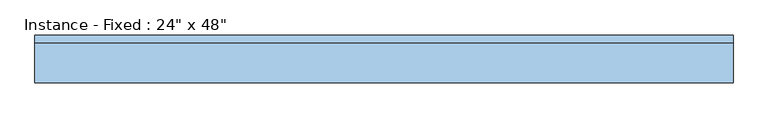
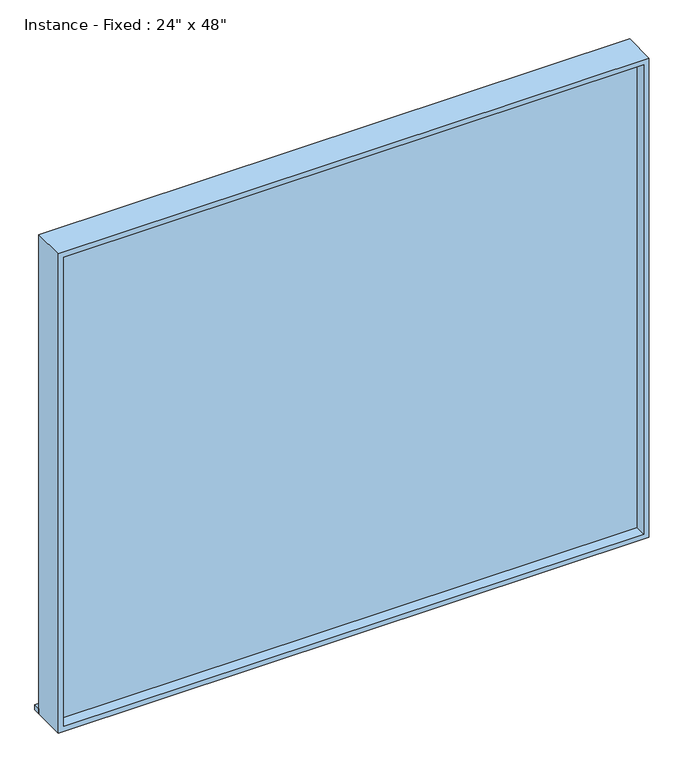
"""IFC4 building model written with IfcOpenShell, lengths in millimetres: window geometry."""

from ifc_helpers import new_model, si_unit, frame, origin, place, context, project, spatial, polyline, outline, extrude, source, transform, mapped, element, save


def window_88b07bfa(model_context):
    return source(origin(), model_context, "Body", "SweptSolid", [
        extrude(outline(polyline([(-1104.9, 127.0), (1028.7, 127.0), (1028.7, 101.6), (-1104.9, 101.6), (-1104.9, 127.0)])), frame((0.0, 0.0, 914.4), z_axis=(0.0, 0.0, 1.0), x_axis=(1.0, 0.0, 0.0)), (0.0, 0.0, 1.0), 19.05),
        extrude(outline(polyline([(1009.65, 22.225), (-1085.85, 22.225), (-1085.85, 34.925), (1009.65, 34.925), (1009.65, 22.225)])), frame((0.0, 0.0, 933.45), z_axis=(0.0, 0.0, 1.0), x_axis=(1.0, 0.0, 0.0)), (0.0, 0.0, 1.0), 1790.7),
        extrude(outline(polyline([(2743.2, 1028.7), (2743.2, -1104.9), (914.4, -1104.9), (914.4, 1028.7), (2743.2, 1028.7)]), holes=[polyline([(2724.15, 1009.65), (933.45, 1009.65), (933.45, -1085.85), (2724.15, -1085.85), (2724.15, 1009.65)])]), frame((0.0, -19.05, 0.0), z_axis=(0.0, 1.0, 0.0), x_axis=(0.0, 0.0, 1.0)), (0.0, 0.0, 1.0), 120.65),
    ])


if __name__ == "__main__":
    model = new_model("IFC4")
    model_context = context("Model", 3, world=origin())
    ifc_project = project(units=[si_unit("LENGTHUNIT", "METRE", prefix="MILLI")], contexts=[model_context])
    site = spatial("IfcSite", under=ifc_project)
    building = spatial("IfcBuilding", under=site)
    placement = place(None, origin())
    window_shape = window_88b07bfa(model_context)
    element("IfcWindow", 1, ObjectType="Instance - Fixed : 24\" x 48\"", at=placement, inside=building, context=model_context, shape_type="MappedRepresentation", body=[
        mapped(window_shape, transform((0.0, 0.0, 0.0), x_axis=(1.0, 0.0, 0.0), y_axis=(0.0, 1.0, 0.0), z_axis=(0.0, 0.0, 1.0))),
    ])
    save(model, "model.ifc")

# Revit data of these elements
# Type "Instance - Fixed : 24\" x 48\""
#   Type Mark = "10"
#   Construction Type Id = "GSP4R"
#   Assembly Code = "B2020100"
#   Analytic Construction = "1/8 in Pilkington single glazing"
#   Visual Light Transmittance = 0.9
#   Thermal Resistance (R) = 0.8466 (h·ft²·°F)/BTU
#   Solar Heat Gain Coefficient = 0.86
#   Heat Transfer Coefficient (U) = 1.1812 BTU/(h·ft²·°F)
#   Height [instance default] = 4' - 0"
#   Default Sill Height = 3' - 0"
#   Width [instance default] = 2' - 0"
#   Window Inset = 0' - 2"
#   Define Thermal Properties by = 1
#   Glass Pane Material = Glass
#   Sash Material = Iron, Ductile
#   Wall Closure = (empty or 0)
# Element 1 (IfcWindow, "Instance - Fixed : 24\" x 48\"")
#   Height = 6' - 0"
#   Width = 7' - 0"
#   Materials on its faces: "Iron, Ductile", "Glass"
# Materials
#   "Glass": class "Glass", colour RGB 0 128 192, transparency 0.75, Description = "Soda Lime Glass", Cost = 0
#   "Iron, Ductile": class "Metal", colour RGB 0 0 0, transparency 0, Description = "Ductile cast iron", Cost = 0
